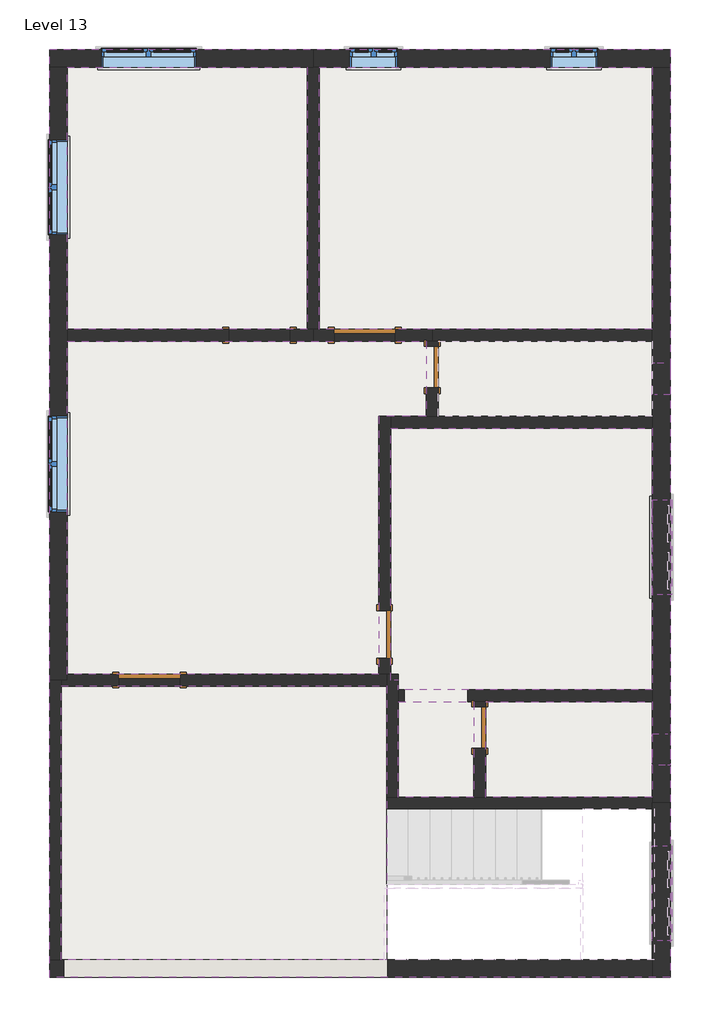
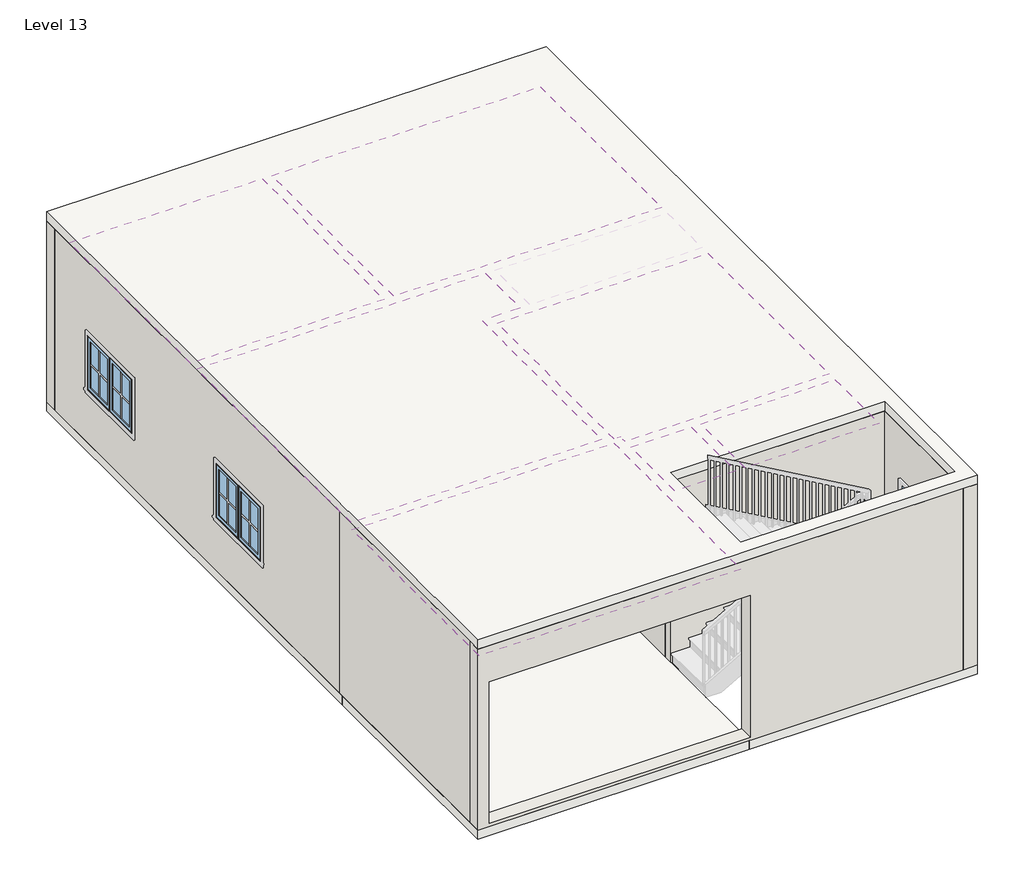
# One storey, part 1 of 2: 27 walls, 13 windows, 7 coverings, 6 doors, 3 slabs.
"""IFC4 building model written with IfcOpenShell, lengths in millimetres."""

from ifc_helpers import new_model, si_unit, frame, origin, place, context, project, spatial, polyline, outline, extrude, faceted_brep, transform, mapped, element, save
from components import door_2908be75, door_9ea4ff49, door_dc34e247, door_b804d09e, fixed_2_415b3208, window_casement_double_3_c417fced, window_casement_double_4_c19c33cb

model = new_model("IFC4")

# Units and contexts
model_context = context("Model", 3, world=origin())
ifc_project = project(units=[si_unit("LENGTHUNIT", "METRE", prefix="MILLI")], contexts=[model_context])

# Site, building, storey
site = spatial("IfcSite", under=ifc_project)
building = spatial("IfcBuilding", under=site)
storey = spatial("IfcBuildingStorey", under=building, Name="Level 13", Elevation=3200.4)

# Coverings
placement = place(None, origin())
element("IfcCovering", 1, ObjectType="2' x 4' ACT System", at=placement, inside=storey, context=model_context, shape_type="SweptSolid", body=[
    extrude(outline(polyline([(-5680.5154463, 2323.8455275), (-5680.5154463, 5678.2330275), (-2607.1154463, 5678.2330275), (-2607.1154463, 2323.8455275), (-5680.5154463, 2323.8455275)])), frame((0.0, 0.0, 5943.6), z_axis=(0.0, 0.0, 1.0), x_axis=(1.0, 0.0, 0.0)), (0.0, 0.0, 1.0), 57.15),
])
element("IfcCovering", 2, ObjectType="2' x 4' ACT System", at=placement, inside=storey, context=model_context, shape_type="SweptSolid", body=[
    extrude(outline(polyline([(-2454.7154463, 2323.8455275), (-2454.7154463, 5678.2330275), (1812.4845537, 5678.2330275), (1812.4845537, 2323.8455275), (-2454.7154463, 2323.8455275)])), frame((0.0, 0.0, 5943.6), z_axis=(0.0, 0.0, 1.0), x_axis=(1.0, 0.0, 0.0)), (0.0, 0.0, 1.0), 57.15),
])
element("IfcCovering", 3, ObjectType="2' x 4' ACT System", at=placement, inside=storey, context=model_context, shape_type="SweptSolid", body=[
    extrude(outline(polyline([(-5680.5154463, -2095.7544725), (-5680.5154463, 2171.4455275), (-1083.1154463, 2171.4455275), (-1083.1154463, 1206.2455275), (-1692.7154463, 1206.2455275), (-1692.7154463, -2095.7544725), (-5680.5154463, -2095.7544725)])), frame((0.0, 0.0, 5943.6), z_axis=(0.0, 0.0, 1.0), x_axis=(1.0, 0.0, 0.0)), (0.0, 0.0, 1.0), 57.15),
])
element("IfcCovering", 4, ObjectType="2' x 4' ACT System", at=placement, inside=storey, context=model_context, shape_type="SweptSolid", body=[
    extrude(outline(polyline([(1812.4845537, 1053.8455275), (1812.4845537, -2298.9544725), (-1438.7154463, -2298.9544725), (-1438.7154463, -2171.9544725), (-1540.3154463, -2171.9544725), (-1540.3154463, 1053.8455275), (1812.4845537, 1053.8455275)])), frame((0.0, 0.0, 5943.6), z_axis=(0.0, 0.0, 1.0), x_axis=(1.0, 0.0, 0.0)), (0.0, 0.0, 1.0), 57.15),
])
element("IfcCovering", 5, ObjectType="2' x 4' ACT System", at=placement, inside=storey, context=model_context, shape_type="SweptSolid", body=[
    extrude(outline(polyline([(1812.4845537, -2451.3544725), (1812.4845537, -3670.5544725), (-321.1154463, -3670.5544725), (-321.1154463, -2451.3544725), (1812.4845537, -2451.3544725)])), frame((0.0, 0.0, 5943.6), z_axis=(0.0, 0.0, 1.0), x_axis=(1.0, 0.0, 0.0)), (0.0, 0.0, 1.0), 57.15),
])
element("IfcCovering", 6, ObjectType="2' x 4' ACT System", at=placement, inside=storey, context=model_context, shape_type="SweptSolid", body=[
    extrude(outline(polyline([(-473.5154463, -2451.3544725), (-473.5154463, -3670.5544725), (-1438.7154463, -3670.5544725), (-1438.7154463, -2451.3544725), (-473.5154463, -2451.3544725)])), frame((0.0, 0.0, 5943.6), z_axis=(0.0, 0.0, 1.0), x_axis=(1.0, 0.0, 0.0)), (0.0, 0.0, 1.0), 57.15),
])
element("IfcCovering", 7, ObjectType="2' x 4' ACT System", at=placement, inside=storey, context=model_context, shape_type="SweptSolid", body=[
    extrude(outline(polyline([(-1591.1154463, -2248.1544725), (-1591.1154463, -5753.3544725), (-5756.7154463, -5753.3544725), (-5756.7154463, -2248.1544725), (-1591.1154463, -2248.1544725)])), frame((0.0, 0.0, 5943.6), z_axis=(0.0, 0.0, 1.0), x_axis=(1.0, 0.0, 0.0)), (0.0, 0.0, 1.0), 57.15),
])

# Doors
door_shape = door_2908be75(model_context)
element("IfcDoor", 8, ObjectType="Single-Flush : 1' 9\"", at=placement, inside=storey, context=model_context, shape_type="MappedRepresentation", body=[
    mapped(door_shape, transform((-397.3154463, -2781.5544725, 3200.4), x_axis=(0.0, 1.0, 0.0), y_axis=(-1.0, 0.0, 0.0), z_axis=(0.0, 0.0, 1.0))),
])
element("IfcDoor", 9, ObjectType="Single-Flush : 1' 9\"", at=placement, inside=storey, context=model_context, shape_type="MappedRepresentation", body=[
    mapped(door_shape, transform((-1006.9154463, 1841.2455275, 3200.4), x_axis=(0.0, 1.0, 0.0), y_axis=(-1.0, 0.0, 0.0), z_axis=(0.0, 0.0, 1.0))),
])
door_2_shape = door_9ea4ff49(model_context)
element("IfcDoor", 10, ObjectType="Single-Flush : 2'0\"", at=placement, inside=storey, context=model_context, shape_type="MappedRepresentation", body=[
    mapped(door_2_shape, transform((-1616.5154463, -1587.7544725, 3200.4), x_axis=(0.0, -1.0, 0.0), y_axis=(1.0, 0.0, 0.0), z_axis=(0.0, 0.0, 1.0))),
])
door_3_shape = door_dc34e247(model_context)
element("IfcDoor", 11, ObjectType="Single-Flush : 2'7\"", at=placement, inside=storey, context=model_context, shape_type="MappedRepresentation", body=[
    mapped(door_3_shape, transform((-4626.4154463, -2171.9544725, 3200.4), x_axis=(-1.0, 0.0, 0.0), y_axis=(0.0, -1.0, 0.0), z_axis=(0.0, 0.0, 1.0))),
])
element("IfcDoor", 12, ObjectType="Single-Flush : 2'7\"", at=placement, inside=storey, context=model_context, shape_type="MappedRepresentation", body=[
    mapped(door_3_shape, transform((-1870.5154463, 2247.6455275, 3200.4), x_axis=(-1.0, 0.0, 0.0), y_axis=(0.0, -1.0, 0.0), z_axis=(0.0, 0.0, 1.0))),
])
door_4_shape = door_b804d09e(model_context)
element("IfcDoor", 13, ObjectType="Single-Flush : 2'7\"", at=placement, inside=storey, context=model_context, shape_type="MappedRepresentation", body=[
    mapped(door_4_shape, transform((-3216.7154463, 2247.6455275, 3200.4), x_axis=(1.0, 0.0, 0.0), y_axis=(0.0, 1.0, 0.0), z_axis=(0.0, 0.0, 1.0))),
])

# Slabs
element("IfcSlab", 14, ObjectType="Generic - 6\"", at=placement, inside=storey, context=model_context, shape_type="SweptSolid", body=[
    extrude(outline(polyline([(-5909.1154463, -2248.1544725), (-5909.1154463, 5906.8330275), (2041.0845537, 5906.8330275), (2041.0845537, -5981.9544725), (-1591.1154463, -5981.9544725), (-1591.1154463, -5753.3544725), (1812.4845537, -5753.3544725), (1812.4845537, -3822.9544725), (-1591.1154463, -3822.9544725), (-1591.1154463, -2248.1544725), (-5756.7154463, -2248.1544725), (-5909.1154463, -2248.1544725)])), frame((0.0, 0.0, 3048.0), z_axis=(0.0, 0.0, 1.0), x_axis=(1.0, 0.0, 0.0)), (0.0, 0.0, 1.0), 152.4),
])
element("IfcSlab", 15, ObjectType="Generic - 6\"", at=placement, inside=storey, context=model_context, shape_type="SweptSolid", body=[
    extrude(outline(polyline([(-1591.1154463, -2248.1544725), (-1591.1154463, -5981.9544725), (-5909.1154463, -5981.9544725), (-5909.1154463, -2248.1544725), (-1591.1154463, -2248.1544725)])), frame((0.0, 0.0, 3048.0), z_axis=(0.0, 0.0, 1.0), x_axis=(1.0, 0.0, 0.0)), (0.0, 0.0, 1.0), 152.4),
])
element("IfcSlab", 16, ObjectType="Generic - 6\"", at=placement, inside=storey, context=model_context, shape_type="SweptSolid", body=[
    extrude(outline(polyline([(2041.0845537, 5906.8330275), (2041.0845537, -5981.9544725), (-5909.1154463, -5981.9544725), (-5909.1154463, 5906.8330275), (2041.0845537, 5906.8330275)]), holes=[polyline([(1812.4845537, -3822.9544725), (-1591.1154463, -3822.9544725), (-1591.1154463, -5753.3544725), (1812.4845537, -5753.3544725), (1812.4845537, -3822.9544725)])]), frame((0.0, 0.0, 6248.4), z_axis=(0.0, 0.0, 1.0), x_axis=(1.0, 0.0, 0.0)), (0.0, 0.0, 1.0), 152.4),
])

# Walls
element("IfcWall", 17, ObjectType="Generic - 6\"", at=placement, inside=storey, context=model_context, shape_type="Brep", body=[
    faceted_brep([(-5909.1154463, -2171.9544725, 3200.4), (-5909.1154463, -5753.3544725, 3200.4), (-5909.1154463, -5753.3544725, 6248.4), (-5909.1154463, -2171.9544725, 6248.4), (-5756.7154463, -2171.9544725, 3200.4), (-5756.7154463, -2171.9544725, 6248.4), (-5756.7154463, -2248.1544725, 6248.4), (-5756.7154463, -5753.3544725, 6248.4), (-5756.7154463, -5753.3544725, 3200.4), (-5756.7154463, -2248.1544725, 3200.4)], [[[0, 1, 2, 3]], [[4, 5, 6, 7, 8, 9]], [[1, 0, 4, 9, 8]], [[3, 2, 7, 6, 5]], [[0, 3, 5, 4]], [[2, 1, 8, 7]]]),
])
element("IfcWall", 18, ObjectType="Generic - 6\"", at=placement, inside=storey, context=model_context, shape_type="Brep", body=[
    faceted_brep([(1812.4845537, -3670.5544725, 3200.4), (-321.1154463, -3670.5544725, 3200.4), (-473.5154463, -3670.5544725, 3200.4), (-1438.7154463, -3670.5544725, 3200.4), (-1591.1154463, -3670.5544725, 3200.4), (-1591.1154463, -3670.5544725, 6248.4), (-1438.7154463, -3670.5544725, 6248.4), (-473.5154463, -3670.5544725, 6248.4), (-321.1154463, -3670.5544725, 6248.4), (1812.4845537, -3670.5544725, 6248.4), (1812.4845537, -3822.9544725, 3200.4), (1812.4845537, -3822.9544725, 6248.4), (-1591.1154463, -3822.9544725, 6248.4), (-1591.1154463, -3822.9544725, 3200.4), (1812.4845537, -3746.7544725, 3200.4), (1812.4845537, -3746.7544725, 6248.4)], [[[0, 1, 2, 3, 4, 5, 6, 7, 8, 9]], [[10, 11, 12, 13]], [[4, 3, 2, 1, 0, 14, 10, 13]], [[9, 8, 7, 6, 5, 12, 11, 15]], [[5, 4, 13, 12]], [[0, 9, 15, 11, 10, 14]]]),
])
element("IfcWall", 19, ObjectType="Generic - 6\"", at=placement, inside=storey, context=model_context, shape_type="Brep", body=[
    faceted_brep([(-1438.7154463, -3670.5544725, 3200.4), (-1438.7154463, -2451.3544725, 3200.4), (-1438.7154463, -2298.9544725, 3200.4), (-1438.7154463, -2095.7544725, 3200.4), (-1438.7154463, -2095.7544725, 6248.4), (-1438.7154463, -2298.9544725, 6248.4), (-1438.7154463, -2451.3544725, 6248.4), (-1438.7154463, -3670.5544725, 6248.4), (-1591.1154463, -3670.5544725, 3200.4), (-1591.1154463, -3670.5544725, 6248.4), (-1591.1154463, -2248.1544725, 6248.4), (-1591.1154463, -2171.9544725, 6248.4), (-1591.1154463, -2095.7544725, 6248.4), (-1591.1154463, -2095.7544725, 3200.4), (-1591.1154463, -2171.9544725, 3200.4), (-1591.1154463, -2248.1544725, 3200.4), (-1540.3154463, -2095.7544725, 3200.4), (-1540.3154463, -2095.7544725, 6248.4)], [[[0, 1, 2, 3, 4, 5, 6, 7]], [[8, 9, 10, 11, 12, 13, 14, 15]], [[3, 2, 1, 0, 8, 15, 14, 13, 16]], [[7, 6, 5, 4, 17, 12, 11, 10, 9]], [[0, 7, 9, 8]], [[4, 3, 16, 13, 12, 17]]]),
])
element("IfcWall", 20, ObjectType="Generic - 6\"", at=placement, inside=storey, context=model_context, shape_type="Brep", body=[
    faceted_brep([(-5020.1154463, -2095.7544725, 5334.0), (-5020.1154463, -2095.7544725, 3200.4), (-5680.5154463, -2095.7544725, 3200.4), (-5680.5154463, -2095.7544725, 6248.4), (-1692.7154463, -2095.7544725, 6248.4), (-1591.1154463, -2095.7544725, 6248.4), (-1591.1154463, -2095.7544725, 3200.4), (-1692.7154463, -2095.7544725, 3200.4), (-4232.7154463, -2095.7544725, 3200.4), (-4232.7154463, -2095.7544725, 5334.0), (-5756.7154463, -2248.1544725, 3200.4), (-5020.1154463, -2248.1544725, 3200.4), (-5020.1154463, -2248.1544725, 5334.0), (-4232.7154463, -2248.1544725, 5334.0), (-4232.7154463, -2248.1544725, 3200.4), (-1591.1154463, -2248.1544725, 3200.4), (-1591.1154463, -2248.1544725, 6248.4), (-5756.7154463, -2248.1544725, 6248.4), (-5756.7154463, -2171.9544725, 3200.4), (-5680.5154463, -2171.9544725, 3200.4), (-5680.5154463, -2171.9544725, 6248.4), (-5756.7154463, -2171.9544725, 6248.4)], [[[0, 1, 2, 3, 4, 5, 6, 7, 8, 9]], [[10, 11, 12, 13, 14, 15, 16, 17]], [[2, 1, 11, 10, 18, 19]], [[8, 7, 6, 15, 14]], [[5, 4, 3, 20, 21, 17, 16]], [[3, 2, 19, 20]], [[19, 18, 21, 20]], [[18, 10, 17, 21]], [[6, 5, 16, 15]], [[12, 11, 1, 0]], [[13, 12, 0, 9]], [[14, 13, 9, 8]]]),
])
element("IfcWall", 21, ObjectType="Generic - 6\"", at=placement, inside=storey, context=model_context, shape_type="Brep", body=[
    faceted_brep([(1812.4845537, -2451.3544725, 3200.4), (1812.4845537, -2451.3544725, 6248.4), (-321.1154463, -2451.3544725, 6248.4), (-473.5154463, -2451.3544725, 6248.4), (-1438.7154463, -2451.3544725, 6248.4), (-1438.7154463, -2451.3544725, 3200.4), (-1367.0206652, -2451.3544725, 3200.4), (-1367.0206652, -2451.3544725, 5638.8), (-547.4818767, -2451.3544725, 5638.8), (-547.4818767, -2451.3544725, 3200.4), (-473.5154463, -2451.3544725, 3200.4), (-321.1154463, -2451.3544725, 3200.4), (1812.4845537, -2298.9544725, 6248.4), (1812.4845537, -2298.9544725, 3200.4), (-547.4818767, -2298.9544725, 3200.4), (-547.4818767, -2298.9544725, 5638.8), (-1367.0206652, -2298.9544725, 5638.8), (-1367.0206652, -2298.9544725, 3200.4), (-1438.7154463, -2298.9544725, 3200.4), (-1438.7154463, -2298.9544725, 6248.4)], [[[0, 1, 2, 3, 4, 5, 6, 7, 8, 9, 10, 11]], [[12, 13, 14, 15, 16, 17, 18, 19]], [[5, 18, 17, 6]], [[13, 0, 11, 10, 9, 14]], [[4, 3, 2, 1, 12, 19]], [[1, 0, 13, 12]], [[5, 4, 19, 18]], [[7, 16, 15, 8]], [[16, 7, 6, 17]], [[8, 15, 14, 9]]]),
])
element("IfcWall", 22, ObjectType="Generic - 6\"", at=placement, inside=storey, context=model_context, shape_type="SweptSolid", body=[
    extrude(outline(polyline([(-2451.3544725, 3200.4), (-2514.8544725, 3200.4), (-2514.8544725, 5334.0), (-3048.2544725, 5334.0), (-3048.2544725, 3200.4), (-3670.5544725, 3200.4), (-3670.5544725, 6248.4), (-2451.3544725, 6248.4), (-2451.3544725, 3200.4)])), frame((-473.5154463, 0.0, 0.0), z_axis=(1.0, 0.0, 0.0), x_axis=(0.0, 1.0, 0.0)), (0.0, 0.0, 1.0), 152.4),
])
element("IfcWall", 23, ObjectType="Generic - 6\"", at=placement, inside=storey, context=model_context, shape_type="Brep", body=[
    faceted_brep([(-1540.3154463, -2095.7544725, 3200.4), (-1540.3154463, -1892.5544725, 3200.4), (-1540.3154463, -1892.5544725, 5334.0), (-1540.3154463, -1282.9544725, 5334.0), (-1540.3154463, -1282.9544725, 3200.4), (-1540.3154463, 1053.8455275, 3200.4), (-1540.3154463, 1206.2455275, 3200.4), (-1540.3154463, 1206.2455275, 6248.4), (-1540.3154463, 1053.8455275, 6248.4), (-1540.3154463, -2095.7544725, 6248.4), (-1692.7154463, -1892.5544725, 5334.0), (-1692.7154463, -1892.5544725, 3200.4), (-1692.7154463, -2095.7544725, 3200.4), (-1692.7154463, -2095.7544725, 6248.4), (-1692.7154463, 1206.2455275, 6248.4), (-1692.7154463, 1206.2455275, 3200.4), (-1692.7154463, -1282.9544725, 3200.4), (-1692.7154463, -1282.9544725, 5334.0), (-1591.1154463, -2095.7544725, 3200.4), (-1591.1154463, -2095.7544725, 6248.4)], [[[0, 1, 2, 3, 4, 5, 6, 7, 8, 9]], [[10, 11, 12, 13, 14, 15, 16, 17]], [[16, 15, 6, 5, 4]], [[12, 11, 1, 0, 18]], [[9, 8, 7, 14, 13, 19]], [[0, 9, 19, 13, 12, 18]], [[7, 6, 15, 14]], [[2, 1, 11, 10]], [[3, 2, 10, 17]], [[4, 3, 17, 16]]]),
])
element("IfcWall", 24, ObjectType="Generic - 6\"", at=placement, inside=storey, context=model_context, shape_type="Brep", body=[
    faceted_brep([(-1540.3154463, 1053.8455275, 3200.4), (1812.4845537, 1053.8455275, 3200.4), (1812.4845537, 1053.8455275, 6248.4), (-1540.3154463, 1053.8455275, 6248.4), (-1540.3154463, 1206.2455275, 3200.4), (-1540.3154463, 1206.2455275, 6248.4), (-1083.1154463, 1206.2455275, 6248.4), (-930.7154463, 1206.2455275, 6248.4), (1812.4845537, 1206.2455275, 6248.4), (1812.4845537, 1206.2455275, 3200.4), (-930.7154463, 1206.2455275, 3200.4), (-1083.1154463, 1206.2455275, 3200.4)], [[[0, 1, 2, 3]], [[4, 5, 6, 7, 8, 9, 10, 11]], [[1, 0, 4, 11, 10, 9]], [[3, 2, 8, 7, 6, 5]], [[0, 3, 5, 4]], [[2, 1, 9, 8]]]),
])
element("IfcWall", 25, ObjectType="Generic - 6\"", at=placement, inside=storey, context=model_context, shape_type="Brep", body=[
    faceted_brep([(-930.7154463, 2107.9455275, 5334.0), (-930.7154463, 2107.9455275, 3200.4), (-930.7154463, 2171.4455275, 3200.4), (-930.7154463, 2171.4455275, 6248.4), (-930.7154463, 1206.2455275, 6248.4), (-930.7154463, 1206.2455275, 3200.4), (-930.7154463, 1574.5455275, 3200.4), (-930.7154463, 1574.5455275, 5334.0), (-1083.1154463, 2171.4455275, 3200.4), (-1083.1154463, 2107.9455275, 3200.4), (-1083.1154463, 2107.9455275, 5334.0), (-1083.1154463, 1574.5455275, 5334.0), (-1083.1154463, 1574.5455275, 3200.4), (-1083.1154463, 1206.2455275, 3200.4), (-1083.1154463, 1206.2455275, 6248.4), (-1083.1154463, 2171.4455275, 6248.4), (-1006.9154463, 2171.4455275, 3200.4), (-1006.9154463, 2171.4455275, 6248.4)], [[[0, 1, 2, 3, 4, 5, 6, 7]], [[8, 9, 10, 11, 12, 13, 14, 15]], [[6, 5, 13, 12]], [[2, 1, 9, 8, 16]], [[4, 3, 17, 15, 14]], [[5, 4, 14, 13]], [[10, 9, 1, 0]], [[11, 10, 0, 7]], [[12, 11, 7, 6]], [[3, 2, 16, 8, 15, 17]]]),
])
element("IfcWall", 26, ObjectType="Generic - 6\"", at=placement, inside=storey, context=model_context, shape_type="Brep", body=[
    faceted_brep([(1812.4845537, 2323.8455275, 3200.4), (-1006.9154463, 2323.8455275, 3200.4), (-1006.9154463, 2323.8455275, 6248.4), (1812.4845537, 2323.8455275, 6248.4), (1812.4845537, 2171.4455275, 3200.4), (1812.4845537, 2171.4455275, 6248.4), (-930.7154463, 2171.4455275, 6248.4), (-1006.9154463, 2171.4455275, 6248.4), (-1006.9154463, 2171.4455275, 3200.4), (-930.7154463, 2171.4455275, 3200.4)], [[[0, 1, 2, 3]], [[4, 5, 6, 7, 8, 9]], [[1, 0, 4, 9, 8]], [[2, 1, 8, 7]], [[3, 2, 7, 6, 5]], [[0, 3, 5, 4]]]),
])
element("IfcWall", 27, ObjectType="Generic - 6\"", at=placement, inside=storey, context=model_context, shape_type="Brep", body=[
    faceted_brep([(-2607.1154463, 5678.2330275, 3200.4), (-2607.1154463, 2323.8455275, 3200.4), (-2607.1154463, 2323.8455275, 6248.4), (-2607.1154463, 5678.2330275, 6248.4), (-2454.7154463, 5678.2330275, 3200.4), (-2454.7154463, 5678.2330275, 6248.4), (-2454.7154463, 2323.8455275, 6248.4), (-2454.7154463, 2323.8455275, 3200.4), (-2530.9154463, 5678.2330275, 3200.4), (-2530.9154463, 2323.8455275, 3200.4), (-2530.9154463, 2323.8455275, 6248.4), (-2530.9154463, 5678.2330275, 6248.4)], [[[0, 1, 2, 3]], [[4, 5, 6, 7]], [[1, 0, 8, 4, 7, 9]], [[3, 2, 10, 6, 5, 11]], [[0, 3, 11, 5, 4, 8]], [[2, 1, 9, 7, 6, 10]]]),
])
element("IfcWall", 28, ObjectType="Generic - 6\"", at=placement, inside=storey, context=model_context, shape_type="Brep", body=[
    faceted_brep([(-2530.9154463, 2323.8455275, 3200.4), (-2607.1154463, 2323.8455275, 3200.4), (-2823.0154463, 2323.8455275, 3200.4), (-2823.0154463, 2323.8455275, 5334.0), (-3610.4154463, 2323.8455275, 5334.0), (-3610.4154463, 2323.8455275, 3200.4), (-5680.5154463, 2323.8455275, 3200.4), (-5680.5154463, 2323.8455275, 6248.4), (-2607.1154463, 2323.8455275, 6248.4), (-2530.9154463, 2323.8455275, 6248.4), (-2823.0154463, 2171.4455275, 5334.0), (-2823.0154463, 2171.4455275, 3200.4), (-2530.9154463, 2171.4455275, 3200.4), (-2530.9154463, 2171.4455275, 6248.4), (-5680.5154463, 2171.4455275, 6248.4), (-5680.5154463, 2171.4455275, 3200.4), (-3610.4154463, 2171.4455275, 3200.4), (-3610.4154463, 2171.4455275, 5334.0)], [[[0, 1, 2, 3, 4, 5, 6, 7, 8, 9]], [[10, 11, 12, 13, 14, 15, 16, 17]], [[16, 15, 6, 5]], [[12, 11, 2, 1, 0]], [[9, 8, 7, 14, 13]], [[0, 9, 13, 12]], [[7, 6, 15, 14]], [[5, 4, 17, 16]], [[4, 3, 10, 17]], [[3, 2, 11, 10]]]),
])
element("IfcWall", 29, ObjectType="Generic - 6\"", at=placement, inside=storey, context=model_context, shape_type="Brep", body=[
    faceted_brep([(-2264.2154463, 2323.8455275, 5334.0), (-2264.2154463, 2323.8455275, 3200.4), (-2454.7154463, 2323.8455275, 3200.4), (-2530.9154463, 2323.8455275, 3200.4), (-2530.9154463, 2323.8455275, 6248.4), (-2454.7154463, 2323.8455275, 6248.4), (-1006.9154463, 2323.8455275, 6248.4), (-1006.9154463, 2323.8455275, 3200.4), (-1476.8154463, 2323.8455275, 3200.4), (-1476.8154463, 2323.8455275, 5334.0), (-2530.9154463, 2171.4455275, 3200.4), (-2264.2154463, 2171.4455275, 3200.4), (-2264.2154463, 2171.4455275, 5334.0), (-1476.8154463, 2171.4455275, 5334.0), (-1476.8154463, 2171.4455275, 3200.4), (-1083.1154463, 2171.4455275, 3200.4), (-1006.9154463, 2171.4455275, 3200.4), (-1006.9154463, 2171.4455275, 6248.4), (-1083.1154463, 2171.4455275, 6248.4), (-2530.9154463, 2171.4455275, 6248.4)], [[[0, 1, 2, 3, 4, 5, 6, 7, 8, 9]], [[10, 11, 12, 13, 14, 15, 16, 17, 18, 19]], [[8, 7, 16, 15, 14]], [[3, 2, 1, 11, 10]], [[4, 3, 10, 19]], [[6, 5, 4, 19, 18, 17]], [[7, 6, 17, 16]], [[14, 13, 9, 8]], [[13, 12, 0, 9]], [[12, 11, 1, 0]]]),
])
element("IfcWall", 30, ObjectType="Generic - 6\"", at=placement, inside=storey, context=model_context, shape_type="SweptSolid", body=[
    extrude(outline(polyline([(-5680.5154463, -2095.7544725), (-1692.7154463, -2095.7544725), (-1692.7154463, -2171.9544725), (-1591.1154463, -2171.9544725), (-1591.1154463, -2248.1544725), (-5756.7154463, -2248.1544725), (-5756.7154463, -2171.9544725), (-5680.5154463, -2171.9544725), (-5680.5154463, -2095.7544725)])), frame((0.0, 0.0, 3200.4), z_axis=(0.0, 0.0, 1.0), x_axis=(1.0, 0.0, 0.0)), (0.0, 0.0, 1.0), 3048.0),
])
element("IfcWall", 31, ObjectType="Generic - 6\"", at=placement, inside=storey, context=model_context, shape_type="Brep", body=[
    faceted_brep([(-2607.1154463, 5678.2330275, 3200.4), (-2607.1154463, 2323.8455275, 3200.4), (-2607.1154463, 2323.8455275, 6248.4), (-2607.1154463, 5678.2330275, 6248.4), (-2454.7154463, 5678.2330275, 3200.4), (-2454.7154463, 5678.2330275, 6248.4), (-2454.7154463, 2323.8455275, 6248.4), (-2454.7154463, 2323.8455275, 3200.4), (-2530.9154463, 5678.2330275, 3200.4), (-2530.9154463, 2323.8455275, 3200.4), (-2530.9154463, 2323.8455275, 6248.4), (-2530.9154463, 5678.2330275, 6248.4)], [[[0, 1, 2, 3]], [[4, 5, 6, 7]], [[1, 0, 8, 4, 7, 9]], [[3, 2, 10, 6, 5, 11]], [[0, 3, 11, 5, 4, 8]], [[2, 1, 9, 7, 6, 10]]]),
])
element("IfcWall", 32, ObjectType="Generic - 6\"", at=placement, inside=storey, context=model_context, shape_type="Brep", body=[
    faceted_brep([(-2530.9154463, 2323.8455275, 3200.4), (-2607.1154463, 2323.8455275, 3200.4), (-5680.5154463, 2323.8455275, 3200.4), (-5680.5154463, 2323.8455275, 6248.4), (-2607.1154463, 2323.8455275, 6248.4), (-2530.9154463, 2323.8455275, 6248.4), (-2530.9154463, 2171.4455275, 3200.4), (-2530.9154463, 2171.4455275, 6248.4), (-5680.5154463, 2171.4455275, 6248.4), (-5680.5154463, 2171.4455275, 3200.4)], [[[0, 1, 2, 3, 4, 5]], [[6, 7, 8, 9]], [[2, 1, 0, 6, 9]], [[5, 4, 3, 8, 7]], [[0, 5, 7, 6]], [[3, 2, 9, 8]]]),
])
element("IfcWall", 33, ObjectType="Generic - 6\"", at=placement, inside=storey, context=model_context, shape_type="Brep", body=[
    faceted_brep([(-1006.9154463, 2323.8455275, 3200.4), (-2454.7154463, 2323.8455275, 3200.4), (-2530.9154463, 2323.8455275, 3200.4), (-2530.9154463, 2323.8455275, 6248.4), (-2454.7154463, 2323.8455275, 6248.4), (-1006.9154463, 2323.8455275, 6248.4), (-1006.9154463, 2171.4455275, 3200.4), (-1006.9154463, 2171.4455275, 6248.4), (-1083.1154463, 2171.4455275, 6248.4), (-2530.9154463, 2171.4455275, 6248.4), (-2530.9154463, 2171.4455275, 3200.4), (-1083.1154463, 2171.4455275, 3200.4)], [[[0, 1, 2, 3, 4, 5]], [[6, 7, 8, 9, 10, 11]], [[2, 1, 0, 6, 11, 10]], [[3, 2, 10, 9]], [[5, 4, 3, 9, 8, 7]], [[0, 5, 7, 6]]]),
])
element("IfcWall", 34, ObjectType="Generic - 9\"", at=placement, inside=storey, context=model_context, shape_type="Brep", body=[
    faceted_brep([(-5909.1154463, 5678.2330275, 3200.4), (-5680.5154463, 5678.2330275, 3200.4), (-2607.1154463, 5678.2330275, 3200.4), (-2530.9154463, 5678.2330275, 3200.4), (-2530.9154463, 5678.2330275, 6248.4), (-2607.1154463, 5678.2330275, 6248.4), (-5680.5154463, 5678.2330275, 6248.4), (-5909.1154463, 5678.2330275, 6248.4), (-4029.5154463, 5678.2330275, 5029.2), (-4029.5154463, 5678.2330275, 4114.8), (-5248.7154463, 5678.2330275, 4114.8), (-5248.7154463, 5678.2330275, 5029.2), (-5909.1154463, 5906.8330275, 3200.4), (-5909.1154463, 5906.8330275, 6248.4), (-2530.9154463, 5906.8330275, 6248.4), (-2530.9154463, 5906.8330275, 3200.4), (-4029.5154463, 5906.8330275, 5029.2), (-5248.7154463, 5906.8330275, 5029.2), (-5248.7154463, 5906.8330275, 4114.8), (-4029.5154463, 5906.8330275, 4114.8)], [[[0, 1, 2, 3, 4, 5, 6, 7], [8, 9, 10, 11]], [[12, 13, 14, 15], [16, 17, 18, 19]], [[3, 2, 1, 0, 12, 15]], [[4, 3, 15, 14]], [[7, 6, 5, 4, 14, 13]], [[0, 7, 13, 12]], [[9, 8, 16, 19]], [[10, 9, 19, 18]], [[11, 10, 18, 17]], [[8, 11, 17, 16]]]),
])
element("IfcWall", 35, ObjectType="Generic - 9\"", at=placement, inside=storey, context=model_context, shape_type="Brep", body=[
    faceted_brep([(1812.4845537, 5678.2330275, 3200.4), (1812.4845537, 2323.8455275, 3200.4), (1812.4845537, 2171.4455275, 3200.4), (1812.4845537, 1206.2455275, 3200.4), (1812.4845537, 1053.8455275, 3200.4), (1812.4845537, -2298.9544725, 3200.4), (1812.4845537, -2451.3544725, 3200.4), (1812.4845537, -3670.5544725, 3200.4), (1812.4845537, -3746.7544725, 3200.4), (1812.4845537, -3746.7544725, 6248.4), (1812.4845537, -3670.5544725, 6248.4), (1812.4845537, -2451.3544725, 6248.4), (1812.4845537, -2298.9544725, 6248.4), (1812.4845537, 1053.8455275, 6248.4), (1812.4845537, 1206.2455275, 6248.4), (1812.4845537, 2171.4455275, 6248.4), (1812.4845537, 2323.8455275, 6248.4), (1812.4845537, 5678.2330275, 6248.4), (1812.4845537, -1079.7544725, 5334.0), (1812.4845537, -1079.7544725, 4419.6), (1812.4845537, 139.4455275, 4419.6), (1812.4845537, 139.4455275, 5334.0), (1812.4845537, -3264.1544725, 5638.8), (1812.4845537, -3264.1544725, 5029.2), (1812.4845537, -2857.7544725, 5029.2), (1812.4845537, -2857.7544725, 5638.8), (1812.4845537, 1892.0455275, 5638.8), (1812.4845537, 1485.6455275, 5638.8), (1812.4845537, 1485.6455275, 5029.2), (1812.4845537, 1892.0455275, 5029.2), (2041.0845537, 5678.2330275, 3200.4), (2041.0845537, 5678.2330275, 6248.4), (2041.0845537, -3746.7544725, 6248.4), (2041.0845537, -3746.7544725, 3200.4), (2041.0845537, -1079.7544725, 5334.0), (2041.0845537, 139.4455275, 5334.0), (2041.0845537, 139.4455275, 4419.6), (2041.0845537, -1079.7544725, 4419.6), (2041.0845537, -3264.1544725, 5638.8), (2041.0845537, -2857.7544725, 5638.8), (2041.0845537, -2857.7544725, 5029.2), (2041.0845537, -3264.1544725, 5029.2), (2041.0845537, 1892.0455275, 5638.8), (2041.0845537, 1892.0455275, 5029.2), (2041.0845537, 1485.6455275, 5029.2), (2041.0845537, 1485.6455275, 5638.8)], [[[0, 1, 2, 3, 4, 5, 6, 7, 8, 9, 10, 11, 12, 13, 14, 15, 16, 17], [18, 19, 20, 21], [22, 23, 24, 25], [26, 27, 28, 29]], [[30, 31, 32, 33], [34, 35, 36, 37], [38, 39, 40, 41], [42, 43, 44, 45]], [[8, 7, 6, 5, 4, 3, 2, 1, 0, 30, 33]], [[9, 8, 33, 32]], [[17, 16, 15, 14, 13, 12, 11, 10, 9, 32, 31]], [[0, 17, 31, 30]], [[19, 18, 34, 37]], [[20, 19, 37, 36]], [[21, 20, 36, 35]], [[18, 21, 35, 34]], [[23, 22, 38, 41]], [[24, 23, 41, 40]], [[25, 24, 40, 39]], [[22, 25, 39, 38]], [[43, 42, 26, 29]], [[44, 43, 29, 28]], [[45, 44, 28, 27]], [[42, 45, 27, 26]]]),
])
element("IfcWall", 36, ObjectType="Generic - 9\"", at=placement, inside=storey, context=model_context, shape_type="Brep", body=[
    faceted_brep([(1812.4845537, -5753.3544725, 3200.4), (-5756.7154463, -5753.3544725, 3200.4), (-5909.1154463, -5753.3544725, 3200.4), (-5909.1154463, -5753.3544725, 6248.4), (-5756.7154463, -5753.3544725, 6248.4), (1812.4845537, -5753.3544725, 6248.4), (-1576.8982041, -5753.3544725, 5638.8), (-5729.1673724, -5753.3544725, 5638.8), (-5729.1673724, -5753.3544725, 3251.2), (-1576.8982041, -5753.3544725, 3251.2), (-5909.1154463, -5981.9544725, 3200.4), (1812.4845537, -5981.9544725, 3200.4), (1812.4845537, -5981.9544725, 6248.4), (-5909.1154463, -5981.9544725, 6248.4), (-5729.1673724, -5981.9544725, 5638.8), (-1576.8982041, -5981.9544725, 5638.8), (-1576.8982041, -5981.9544725, 3251.2), (-5729.1673724, -5981.9544725, 3251.2)], [[[0, 1, 2, 3, 4, 5], [6, 7, 8, 9]], [[10, 11, 12, 13], [14, 15, 16, 17]], [[2, 1, 0, 11, 10]], [[5, 4, 3, 13, 12]], [[0, 5, 12, 11]], [[6, 15, 14, 7]], [[8, 17, 16, 9]], [[15, 6, 9, 16]], [[7, 14, 17, 8]], [[3, 2, 10, 13]]]),
])
element("IfcWall", 37, ObjectType="Generic - 9\"", at=placement, inside=storey, context=model_context, shape_type="Brep", body=[
    faceted_brep([(-5909.1154463, 5678.2330275, 3200.4), (-5909.1154463, -2171.9544725, 3200.4), (-5909.1154463, -2171.9544725, 6248.4), (-5909.1154463, 5678.2330275, 6248.4), (-5909.1154463, 4751.1330275, 5029.2), (-5909.1154463, 3531.9330275, 5029.2), (-5909.1154463, 3531.9330275, 4114.8), (-5909.1154463, 4751.1330275, 4114.8), (-5909.1154463, 1206.2455275, 5029.2), (-5909.1154463, -12.9544725, 5029.2), (-5909.1154463, -12.9544725, 4114.8), (-5909.1154463, 1206.2455275, 4114.8), (-5680.5154463, 5678.2330275, 3200.4), (-5680.5154463, 5678.2330275, 6248.4), (-5680.5154463, 2323.8455275, 6248.4), (-5680.5154463, 2171.4455275, 6248.4), (-5680.5154463, -2095.7544725, 6248.4), (-5680.5154463, -2171.9544725, 6248.4), (-5680.5154463, -2171.9544725, 3200.4), (-5680.5154463, -2095.7544725, 3200.4), (-5680.5154463, 2171.4455275, 3200.4), (-5680.5154463, 2323.8455275, 3200.4), (-5680.5154463, 4751.1330275, 5029.2), (-5680.5154463, 4751.1330275, 4114.8), (-5680.5154463, 3531.9330275, 4114.8), (-5680.5154463, 3531.9330275, 5029.2), (-5680.5154463, 1206.2455275, 5029.2), (-5680.5154463, 1206.2455275, 4114.8), (-5680.5154463, -12.9544725, 4114.8), (-5680.5154463, -12.9544725, 5029.2), (-5756.7154463, -2171.9544725, 3200.4), (-5756.7154463, -2171.9544725, 6248.4)], [[[0, 1, 2, 3], [4, 5, 6, 7], [8, 9, 10, 11]], [[12, 13, 14, 15, 16, 17, 18, 19, 20, 21], [22, 23, 24, 25], [26, 27, 28, 29]], [[1, 0, 12, 21, 20, 19, 18, 30]], [[2, 1, 30, 18, 17, 31]], [[3, 2, 31, 17, 16, 15, 14, 13]], [[0, 3, 13, 12]], [[23, 22, 4, 7]], [[24, 23, 7, 6]], [[25, 24, 6, 5]], [[22, 25, 5, 4]], [[27, 26, 8, 11]], [[28, 27, 11, 10]], [[29, 28, 10, 9]], [[26, 29, 9, 8]]]),
])
element("IfcWall", 38, ObjectType="Generic - 9\"", at=placement, inside=storey, context=model_context, shape_type="Brep", body=[
    faceted_brep([(-2530.9154463, 5678.2330275, 3200.4), (-2454.7154463, 5678.2330275, 3200.4), (1812.4845537, 5678.2330275, 3200.4), (2041.0845537, 5678.2330275, 3200.4), (2041.0845537, 5678.2330275, 6248.4), (1812.4845537, 5678.2330275, 6248.4), (-2454.7154463, 5678.2330275, 6248.4), (-2530.9154463, 5678.2330275, 6248.4), (-1451.4154463, 5678.2330275, 5029.2), (-1451.4154463, 5678.2330275, 4114.8), (-2061.0154463, 5678.2330275, 4114.8), (-2061.0154463, 5678.2330275, 5029.2), (1113.9845537, 5678.2330275, 5029.2), (1113.9845537, 5678.2330275, 4114.8), (504.3845537, 5678.2330275, 4114.8), (504.3845537, 5678.2330275, 5029.2), (-2530.9154463, 5906.8330275, 3200.4), (-2530.9154463, 5906.8330275, 6248.4), (2041.0845537, 5906.8330275, 6248.4), (2041.0845537, 5906.8330275, 3200.4), (-1451.4154463, 5906.8330275, 5029.2), (-2061.0154463, 5906.8330275, 5029.2), (-2061.0154463, 5906.8330275, 4114.8), (-1451.4154463, 5906.8330275, 4114.8), (1113.9845537, 5906.8330275, 5029.2), (504.3845537, 5906.8330275, 5029.2), (504.3845537, 5906.8330275, 4114.8), (1113.9845537, 5906.8330275, 4114.8)], [[[0, 1, 2, 3, 4, 5, 6, 7], [8, 9, 10, 11], [12, 13, 14, 15]], [[16, 17, 18, 19], [20, 21, 22, 23], [24, 25, 26, 27]], [[3, 2, 1, 0, 16, 19]], [[7, 6, 5, 4, 18, 17]], [[0, 7, 17, 16]], [[4, 3, 19, 18]], [[8, 11, 21, 20]], [[11, 10, 22, 21]], [[10, 9, 23, 22]], [[9, 8, 20, 23]], [[12, 15, 25, 24]], [[15, 14, 26, 25]], [[14, 13, 27, 26]], [[13, 12, 24, 27]]]),
])
element("IfcWall", 39, ObjectType="Generic - 9\"", at=placement, inside=storey, context=model_context, shape_type="Brep", body=[
    faceted_brep([(1812.4845537, -3746.7544725, 3200.4), (1812.4845537, -3822.9544725, 3200.4), (1812.4845537, -5753.3544725, 3200.4), (1812.4845537, -5981.9544725, 3200.4), (1812.4845537, -5981.9544725, 6248.4), (1812.4845537, -5753.3544725, 6248.4), (1812.4845537, -3822.9544725, 6248.4), (1812.4845537, -3746.7544725, 6248.4), (1812.4845537, -5512.0544725, 5334.0), (1812.4845537, -5512.0544725, 4419.6), (1812.4845537, -4292.8544725, 4419.6), (1812.4845537, -4292.8544725, 5334.0), (2041.0845537, -3746.7544725, 3200.4), (2041.0845537, -3746.7544725, 6248.4), (2041.0845537, -5981.9544725, 6248.4), (2041.0845537, -5981.9544725, 3200.4), (2041.0845537, -5512.0544725, 5334.0), (2041.0845537, -4292.8544725, 5334.0), (2041.0845537, -4292.8544725, 4419.6), (2041.0845537, -5512.0544725, 4419.6)], [[[0, 1, 2, 3, 4, 5, 6, 7], [8, 9, 10, 11]], [[12, 13, 14, 15], [16, 17, 18, 19]], [[3, 2, 1, 0, 12, 15]], [[7, 6, 5, 4, 14, 13]], [[0, 7, 13, 12]], [[4, 3, 15, 14]], [[8, 11, 17, 16]], [[11, 10, 18, 17]], [[10, 9, 19, 18]], [[9, 8, 16, 19]]]),
])
element("IfcWall", 40, ObjectType="Generic - 9\"", at=placement, inside=storey, context=model_context, shape_type="SweptSolid", body=[
    extrude(outline(polyline([(3200.4, -5680.5154463), (3200.4, -2607.1154463), (6248.4, -2607.1154463), (6248.4, -5680.5154463), (3200.4, -5680.5154463)]), holes=[polyline([(5029.2, -4029.5154463), (4114.8, -4029.5154463), (4114.8, -5248.7154463), (5029.2, -5248.7154463), (5029.2, -4029.5154463)])]), frame((0.0, 5678.2330275, 0.0), z_axis=(0.0, 1.0, 0.0), x_axis=(0.0, 0.0, 1.0)), (0.0, 0.0, 1.0), 228.6),
])
element("IfcWall", 41, ObjectType="Generic - 9\"", at=placement, inside=storey, context=model_context, shape_type="Brep", body=[
    faceted_brep([(1812.4845537, -5753.3544725, 3200.4), (-5756.7154463, -5753.3544725, 3200.4), (-5909.1154463, -5753.3544725, 3200.4), (-5909.1154463, -5753.3544725, 6248.4), (-5756.7154463, -5753.3544725, 6248.4), (1812.4845537, -5753.3544725, 6248.4), (-1576.8982041, -5753.3544725, 5638.8), (-5729.1673724, -5753.3544725, 5638.8), (-5729.1673724, -5753.3544725, 3251.2), (-1576.8982041, -5753.3544725, 3251.2), (-5909.1154463, -5981.9544725, 3200.4), (1812.4845537, -5981.9544725, 3200.4), (1812.4845537, -5981.9544725, 6248.4), (-5909.1154463, -5981.9544725, 6248.4), (-5729.1673724, -5981.9544725, 5638.8), (-1576.8982041, -5981.9544725, 5638.8), (-1576.8982041, -5981.9544725, 3251.2), (-5729.1673724, -5981.9544725, 3251.2)], [[[0, 1, 2, 3, 4, 5], [6, 7, 8, 9]], [[10, 11, 12, 13], [14, 15, 16, 17]], [[2, 1, 0, 11, 10]], [[5, 4, 3, 13, 12]], [[6, 15, 14, 7]], [[8, 17, 16, 9]], [[15, 6, 9, 16]], [[7, 14, 17, 8]], [[3, 2, 10, 13]], [[0, 5, 12, 11]]]),
])
element("IfcWall", 42, ObjectType="Generic - 9\"", at=placement, inside=storey, context=model_context, shape_type="SweptSolid", body=[
    extrude(outline(polyline([(3200.4, -2454.7154463), (3200.4, 1812.4845537), (6248.4, 1812.4845537), (6248.4, -2454.7154463), (3200.4, -2454.7154463)]), holes=[polyline([(5029.2, -1451.4154463), (4114.8, -1451.4154463), (4114.8, -2061.0154463), (5029.2, -2061.0154463), (5029.2, -1451.4154463)]), polyline([(5029.2, 1113.9845537), (4114.8, 1113.9845537), (4114.8, 504.3845537), (5029.2, 504.3845537), (5029.2, 1113.9845537)])]), frame((0.0, 5678.2330275, 0.0), z_axis=(0.0, 1.0, 0.0), x_axis=(0.0, 0.0, 1.0)), (0.0, 0.0, 1.0), 228.6),
])
element("IfcWall", 43, ObjectType="Generic - 9\"", at=placement, inside=storey, context=model_context, shape_type="SweptSolid", body=[
    extrude(outline(polyline([(-3822.9544725, 3200.4), (-5753.3544725, 3200.4), (-5753.3544725, 6248.4), (-3822.9544725, 6248.4), (-3822.9544725, 3200.4)]), holes=[polyline([(-5512.0544725, 5334.0), (-5512.0544725, 4419.6), (-4292.8544725, 4419.6), (-4292.8544725, 5334.0), (-5512.0544725, 5334.0)])]), frame((1812.4845537, 0.0, 0.0), z_axis=(1.0, 0.0, 0.0), x_axis=(0.0, 1.0, 0.0)), (0.0, 0.0, 1.0), 228.6),
])

# Windows
fixed_2_shape = fixed_2_415b3208(model_context)
element("IfcWindow", 44, ObjectType="Fixed : 2'", at=placement, inside=storey, context=model_context, shape_type="MappedRepresentation", body=[
    mapped(fixed_2_shape, transform((1926.7845537, -3099.0544725, 4724.4), x_axis=(0.0, -1.0, 0.0), y_axis=(1.0, 0.0, 0.0), z_axis=(0.0, 0.0, 1.0))),
])
element("IfcWindow", 45, ObjectType="Fixed : 2'", at=placement, inside=storey, context=model_context, shape_type="MappedRepresentation", body=[
    mapped(fixed_2_shape, transform((1926.7845537, 1726.9455275, 4724.4), x_axis=(0.0, 1.0, 0.0), y_axis=(-1.0, 0.0, 0.0), z_axis=(0.0, 0.0, 1.0))),
])
window_casement_double_3_shape = window_casement_double_3_c417fced(model_context)
element("IfcWindow", 46, ObjectType="Window-Casement-Double : 3'", at=placement, inside=storey, context=model_context, shape_type="MappedRepresentation", body=[
    mapped(window_casement_double_3_shape, transform((-1756.2154463, 5792.5330275, 3200.4), x_axis=(1.0, 0.0, 0.0), y_axis=(0.0, 1.0, 0.0), z_axis=(0.0, 0.0, 1.0))),
])
element("IfcWindow", 47, ObjectType="Window-Casement-Double : 3'", at=placement, inside=storey, context=model_context, shape_type="MappedRepresentation", body=[
    mapped(window_casement_double_3_shape, transform((809.1845537, 5792.5330275, 3200.4), x_axis=(1.0, 0.0, 0.0), y_axis=(0.0, 1.0, 0.0), z_axis=(0.0, 0.0, 1.0))),
])
element("IfcWindow", 48, ObjectType="Window-Casement-Double : 3'", at=placement, inside=storey, context=model_context, shape_type="MappedRepresentation", body=[
    mapped(window_casement_double_3_shape, transform((-1756.2154463, 5792.5330275, 3200.4), x_axis=(1.0, 0.0, 0.0), y_axis=(0.0, 1.0, 0.0), z_axis=(0.0, 0.0, 1.0))),
])
element("IfcWindow", 49, ObjectType="Window-Casement-Double : 3'", at=placement, inside=storey, context=model_context, shape_type="MappedRepresentation", body=[
    mapped(window_casement_double_3_shape, transform((809.1845537, 5792.5330275, 3200.4), x_axis=(1.0, 0.0, 0.0), y_axis=(0.0, 1.0, 0.0), z_axis=(0.0, 0.0, 1.0))),
])
window_casement_double_4_shape = window_casement_double_4_c19c33cb(model_context)
element("IfcWindow", 50, ObjectType="Window-Casement-Double : 4'", at=placement, inside=storey, context=model_context, shape_type="MappedRepresentation", body=[
    mapped(window_casement_double_4_shape, transform((-4639.1154463, 5792.5330275, 3200.4), x_axis=(1.0, 0.0, 0.0), y_axis=(0.0, 1.0, 0.0), z_axis=(0.0, 0.0, 1.0))),
])
element("IfcWindow", 51, ObjectType="Window-Casement-Double : 4'", at=placement, inside=storey, context=model_context, shape_type="MappedRepresentation", body=[
    mapped(window_casement_double_4_shape, transform((-5794.8154463, 4141.5330275, 3200.4), x_axis=(0.0, 1.0, 0.0), y_axis=(-1.0, 0.0, 0.0), z_axis=(0.0, 0.0, 1.0))),
])
element("IfcWindow", 52, ObjectType="Window-Casement-Double : 4'", at=placement, inside=storey, context=model_context, shape_type="MappedRepresentation", body=[
    mapped(window_casement_double_4_shape, transform((-5794.8154463, 596.6455275, 3200.4), x_axis=(0.0, 1.0, 0.0), y_axis=(-1.0, 0.0, 0.0), z_axis=(0.0, 0.0, 1.0))),
])
element("IfcWindow", 53, ObjectType="Window-Casement-Double : 4'", at=placement, inside=storey, context=model_context, shape_type="MappedRepresentation", body=[
    mapped(window_casement_double_4_shape, transform((1926.7845537, -470.1544725, 3505.2), x_axis=(0.0, -1.0, 0.0), y_axis=(1.0, 0.0, 0.0), z_axis=(0.0, 0.0, 1.0))),
])
element("IfcWindow", 54, ObjectType="Window-Casement-Double : 4'", at=placement, inside=storey, context=model_context, shape_type="MappedRepresentation", body=[
    mapped(window_casement_double_4_shape, transform((1926.7845537, -4902.4544725, 3505.2), x_axis=(0.0, -1.0, 0.0), y_axis=(1.0, 0.0, 0.0), z_axis=(0.0, 0.0, 1.0))),
])
element("IfcWindow", 55, ObjectType="Window-Casement-Double : 4'", at=placement, inside=storey, context=model_context, shape_type="MappedRepresentation", body=[
    mapped(window_casement_double_4_shape, transform((-4639.1154463, 5792.5330275, 3200.4), x_axis=(1.0, 0.0, 0.0), y_axis=(0.0, 1.0, 0.0), z_axis=(0.0, 0.0, 1.0))),
])
element("IfcWindow", 56, ObjectType="Window-Casement-Double : 4'", at=placement, inside=storey, context=model_context, shape_type="MappedRepresentation", body=[
    mapped(window_casement_double_4_shape, transform((1926.7845537, -4902.4544725, 3505.2), x_axis=(0.0, -1.0, 0.0), y_axis=(1.0, 0.0, 0.0), z_axis=(0.0, 0.0, 1.0))),
])

save(model, "model.ifc")

# Revit data of these elements
# Type "2' x 4' ACT System"
#   Assembly Code = "C3030210"
#   built-in parameter 1002203 = 1 (stored number, unit not read)
#   built-in parameter 1002202 = 1 (stored number, unit not read)
#   Layers, outside or top first: 0' - 1 5/8" "Default" (function 1); 0' - 0 5/8" "Acoustic Ceiling Tile 24 x 48" (function 5)
# Type "Single-Flush : 1' 9\""
#   Type Mark = "10"
#   Construction Type Id = "MDOOR"
#   Assembly Code = "C1020"
#   Analytic Construction = "Metal"
#   Thickness = 0' - 2"
#   Heat Transfer Coefficient (U) = 0.651978 BTU/(h·ft²·°F)
#   Height = 7' - 0"
#   Trim Projection Ext = 0' - 1"
#   Trim Projection Int = 0' - 1"
#   Trim Width = 0' - 3"
#   Width = 1' - 9"
#   Define Thermal Properties by = 1
#   Door Material = Door - Panel
#   Frame Material = Door - Frame
#   Visual Light Transmittance = 0
#   Solar Heat Gain Coefficient = 0
#   Function = (empty or 0)
#   Wall Closure = (empty or 0)
# Type "Single-Flush : 2'0\""
#   Type Mark = "9"
#   Construction Type Id = "MDOOR"
#   Assembly Code = "C1020"
#   Analytic Construction = "Metal"
#   Thickness = 0' - 2"
#   Heat Transfer Coefficient (U) = 0.651978 BTU/(h·ft²·°F)
#   Height = 7' - 0"
#   Trim Projection Ext = 0' - 1"
#   Trim Projection Int = 0' - 1"
#   Trim Width = 0' - 3"
#   Width = 2' - 0"
#   Define Thermal Properties by = 1
#   Door Material = Door - Panel
#   Frame Material = Door - Frame
#   Visual Light Transmittance = 0
#   Solar Heat Gain Coefficient = 0
#   Function = (empty or 0)
#   Wall Closure = (empty or 0)
# Type "Single-Flush : 2'7\""
#   Type Mark = "8"
#   Construction Type Id = "MDOOR"
#   Assembly Code = "C1020"
#   Analytic Construction = "Metal"
#   Thickness = 0' - 2"
#   Heat Transfer Coefficient (U) = 0.651978 BTU/(h·ft²·°F)
#   Height = 7' - 0"
#   Trim Projection Ext = 0' - 1"
#   Trim Projection Int = 0' - 1"
#   Trim Width = 0' - 3"
#   Width = 2' - 7"
#   Define Thermal Properties by = 1
#   Door Material = Door - Panel
#   Frame Material = Door - Frame
#   Visual Light Transmittance = 0
#   Solar Heat Gain Coefficient = 0
#   Function = (empty or 0)
#   Wall Closure = (empty or 0)
# Type "Generic - 6\""
#   Assembly Code = "B1010"
#   Function = 0
#   Layers, outside or top first: 0' - 6" no material (function 1)
# Type "Generic - 6\""
#   Assembly Code = "B2010"
#   Layers, outside or top first: 0' - 6" no material (function 1)
# Type "Generic - 9\""
#   Assembly Code = "B2010"
#   Layers, outside or top first: 0' - 9" no material (function 1)
# Type "Fixed : 2'"
#   Type Mark = "20"
#   Construction Type Id = "GSP4R"
#   Assembly Code = "B2020100"
#   Analytic Construction = "1/8 in Pilkington single glazing"
#   Visual Light Transmittance = 0.9
#   Solar Heat Gain Coefficient = 0.78
#   Heat Transfer Coefficient (U) = 0.6496 BTU/(h·ft²·°F)
#   Height = 2' - 0"
#   Default Sill Height = 1' - 0"
#   Width = 1' - 4"
#   Window Inset = 0' - 0 3/4"
#   Define Thermal Properties by = 1
#   Glass Pane Material = Glass
#   Sash Material = Sash
#   Wall Closure = (empty or 0)
# Type "Window-Casement-Double : 3'"
#   Type Mark = "19"
#   Fire Rating = "0.5h"
#   Assembly Code = "B2020100"
#   Analytic Construction = "Double glazing - domestic"
#   Frame Extension [instance default] = 0' - 0 1/4"
#   Window Inset [instance default] = 0' - 0"
#   Wall Thickness [instance default] = 0' - 6"
#   Interior Wall Closure [instance default] = 0' - 2 1/4"
#   Half Width = 1' - 0"
#   Visual Light Transmittance = 0.81
#   Thermal Resistance (R) = 1.8146 (h·ft²·°F)/BTU
#   Solar Heat Gain Coefficient = 0.76
#   Rough Width = 2' - 0 1/2"
#   Rough Height = 3' - 0 1/2"
#   Height = 3' - 0"
#   Heat Transfer Coefficient (U) = 0.5511 BTU/(h·ft²·°F)
#   Exterior Wall Closure [instance default] = 0' - 1 1/4"
#   Extension Jamb [instance default] = 0' - 2 1/4"
#   Default Sill Height = 3' - 0"
#   Width = 2' - 0"
#   Muntin Visibility = yes
#   Interior Trim Visibility [instance default] = yes
#   Exterior Trim Visibility [instance default] = yes
#   Extension Jamb Visibility [instance default] = yes
#   Interior Trim Material = Wood - Stained
#   Muntin Pattern = Muntin Pattern_2x2 : Muntin Pattern_2x2
#   Interior Trim = Trim-Window-Interior-Flat : Picture Frame
#   Interior Frame Material = Wood - Stained
#   Glass Panel Material = Glass
#   Exterior Trim Material = Clad - White
#   Exterior Trim = Trim-Window-Exterior-Flat : with Sill
#   Exterior Frame Material = Clad - White
#   Wall Closure = (empty or 0)
# Type "Window-Casement-Double : 4'"
#   Type Mark = "18"
#   Fire Rating = "0.5h"
#   Assembly Code = "B2020100"
#   Analytic Construction = "Double glazing - domestic"
#   Frame Extension [instance default] = 0' - 0 1/4"
#   Window Inset [instance default] = 0' - 0"
#   Wall Thickness [instance default] = 0' - 6"
#   Interior Wall Closure [instance default] = 0' - 2 1/4"
#   Half Width = 2' - 0"
#   Visual Light Transmittance = 0.81
#   Thermal Resistance (R) = 1.8146 (h·ft²·°F)/BTU
#   Solar Heat Gain Coefficient = 0.76
#   Rough Width = 4' - 0 1/2"
#   Rough Height = 3' - 0 1/2"
#   Height = 3' - 0"
#   Heat Transfer Coefficient (U) = 0.5511 BTU/(h·ft²·°F)
#   Exterior Wall Closure [instance default] = 0' - 1 1/4"
#   Extension Jamb [instance default] = 0' - 2 1/4"
#   Default Sill Height = 3' - 0"
#   Width = 4' - 0"
#   Muntin Visibility = yes
#   Interior Trim Visibility [instance default] = yes
#   Exterior Trim Visibility [instance default] = yes
#   Extension Jamb Visibility [instance default] = yes
#   Interior Trim Material = Wood - Stained
#   Muntin Pattern = Muntin Pattern_2x2 : Muntin Pattern_2x2
#   Interior Trim = Trim-Window-Interior-Flat : Picture Frame
#   Interior Frame Material = Wood - Stained
#   Glass Panel Material = Glass
#   Exterior Trim Material = Clad - White
#   Exterior Trim = Trim-Window-Exterior-Flat : with Sill
#   Exterior Frame Material = Clad - White
#   Wall Closure = (empty or 0)
# Elements 1, 2, 3, 4, 5, 6, 7 (IfcCovering, "2' x 4' ACT System")
#   Height Offset From Level = 9' - 0"
#   Phase Created = New Construction
#   Materials on its faces: "Acoustic Ceiling Tile 24 x 48", "Default"
# Elements 8, 9 (IfcDoor, "Single-Flush : 1' 9\"")
#   Phase Created = New Construction
#   Materials on its faces: "Door - Frame", "Door - Panel"
# Element 10 (IfcDoor, "Single-Flush : 2'0\"")
#   Phase Created = New Construction
#   Materials on its faces: "Door - Frame", "Door - Panel"
# Elements 11, 12, 13 (IfcDoor, "Single-Flush : 2'7\"")
#   Phase Created = New Construction
#   Materials on its faces: "Door - Frame", "Door - Panel"
# Element 14 (IfcSlab, "Generic - 6\"")
#   built-in parameter 1001955 = -1.5708 (stored number, unit not read)
#   Height Offset From Level = 0' - 0"
#   Phase Created = New Construction
#   Materials on its faces: "Default Floor", "TILE"
# Element 15 (IfcSlab, "Generic - 6\"")
#   Height Offset From Level = 0' - 0"
#   Phase Created = New Construction
#   Materials on its faces: "Default Floor", "Grass"
# Element 16 (IfcSlab, "Generic - 6\"")
#   Height Offset From Level = 10' - 6"
#   Phase Created = New Construction
#   Materials on its faces: "Default Floor"
# Element 17 (IfcWall, "Generic - 6\"")
#   Top Offset = 0' - 0"
#   Base Offset = 0' - 0"
#   Unconnected Height = 10' - 0"
#   wall height = 10' - 0"
#   Phase Created = New Construction
#   Base Constraint = Level 13
#   Materials on its faces: "Default Wall", "WALL PAINT 4"
# Element 18 (IfcWall, "Generic - 6\"")
#   Top Offset = 0' - 0"
#   Base Offset = 0' - 0"
#   Unconnected Height = 10' - 0"
#   wall height = 10' - 0"
#   Phase Created = New Construction
#   Base Constraint = Level 13
#   Materials on its faces: "Default Wall", "MARBLE", "WALL PAINT 5"
# Element 19 (IfcWall, "Generic - 6\"")
#   Top Offset = 0' - 0"
#   Base Offset = 0' - 0"
#   Unconnected Height = 10' - 0"
#   wall height = 10' - 0"
#   Phase Created = New Construction
#   Base Constraint = Level 13
#   Materials on its faces: "Default Wall", "WALL PAINT 4", "MARBLE"
# Elements 20, 30 (IfcWall, "Generic - 6\"")
#   Top Offset = 0' - 0"
#   Base Offset = 0' - 0"
#   Unconnected Height = 10' - 0"
#   wall height = 10' - 0"
#   Phase Created = New Construction
#   Base Constraint = Level 13
#   Materials on its faces: "Default Wall", "WALL PAINT 2", "MARBLE"
# Elements 21, 24 (IfcWall, "Generic - 6\"")
#   Top Offset = 0' - 0"
#   Base Offset = 0' - 0"
#   Unconnected Height = 10' - 0"
#   wall height = 10' - 0"
#   Phase Created = New Construction
#   Base Constraint = Level 13
#   Materials on its faces: "Default Wall", "WALL PAINT 4", "WALL PAINT 5"
# Element 22 (IfcWall, "Generic - 6\"")
#   Top Offset = 0' - 0"
#   Base Offset = 0' - 0"
#   Unconnected Height = 10' - 0"
#   wall height = 10' - 0"
#   Phase Created = New Construction
#   Base Constraint = Level 13
#   Materials on its faces: "Default Wall", "WALL PAINT 5"
# Element 23 (IfcWall, "Generic - 6\"")
#   Top Offset = 0' - 0"
#   Base Offset = 0' - 0"
#   Unconnected Height = 10' - 0"
#   wall height = 10' - 0"
#   Phase Created = New Construction
#   Base Constraint = Level 13
#   Materials on its faces: "Default Wall", "WALL PAINT 4", "WALL PAINT 2", "WALL PAINT 5"
# Element 25 (IfcWall, "Generic - 6\"")
#   Top Offset = 0' - 0"
#   Base Offset = 0' - 0"
#   Unconnected Height = 10' - 0"
#   wall height = 10' - 0"
#   Phase Created = New Construction
#   Base Constraint = Level 13
#   Materials on its faces: "Default Wall", "WALL PAINT 5", "WALL PAINT 2"
# Element 26 (IfcWall, "Generic - 6\"")
#   Top Offset = 0' - 0"
#   Base Offset = 0' - 0"
#   Unconnected Height = 10' - 0"
#   wall height = 10' - 0"
#   Phase Created = New Construction
#   Base Constraint = Level 13
#   Materials on its faces: "Default Wall", "WALL PAINT 3", "WALL PAINT 5"
# Elements 27, 31 (IfcWall, "Generic - 6\"")
#   Top Offset = 0' - 0"
#   Base Offset = 0' - 0"
#   Unconnected Height = 10' - 0"
#   wall height = 10' - 0"
#   Phase Created = New Construction
#   Base Constraint = Level 13
#   Materials on its faces: "Default Wall", "WALL PAINT 1", "WALL PAINT 3"
# Elements 28, 32 (IfcWall, "Generic - 6\"")
#   Top Offset = 0' - 0"
#   Base Offset = 0' - 0"
#   Unconnected Height = 10' - 0"
#   wall height = 10' - 0"
#   Phase Created = New Construction
#   Base Constraint = Level 13
#   Materials on its faces: "Default Wall", "WALL PAINT 1", "WALL PAINT 2"
# Elements 29, 33 (IfcWall, "Generic - 6\"")
#   Top Offset = 0' - 0"
#   Base Offset = 0' - 0"
#   Unconnected Height = 10' - 0"
#   wall height = 10' - 0"
#   Phase Created = New Construction
#   Base Constraint = Level 13
#   Materials on its faces: "Default Wall", "WALL PAINT 3", "WALL PAINT 2"
# Elements 34, 40 (IfcWall, "Generic - 9\"")
#   Top Offset = 0' - 0"
#   Base Offset = 0' - 0"
#   Unconnected Height = 10' - 0"
#   wall height = 10' - 0"
#   Phase Created = New Construction
#   Base Constraint = Level 13
#   Materials on its faces: "Default Wall", "WALL PAINT 1"
# Elements 35, 37 (IfcWall, "Generic - 9\"")
#   Top Offset = 0' - 0"
#   Base Offset = 0' - 0"
#   Unconnected Height = 10' - 0"
#   wall height = 10' - 0"
#   Phase Created = New Construction
#   Base Constraint = Level 13
#   Materials on its faces: "Default Wall"
# Elements 36, 39, 41, 43 (IfcWall, "Generic - 9\"")
#   Top Offset = 0' - 0"
#   Base Offset = 0' - 0"
#   Unconnected Height = 10' - 0"
#   wall height = 10' - 0"
#   Phase Created = New Construction
#   Base Constraint = Level 13
#   Materials on its faces: "Default Wall", "WALL PAINT 4"
# Elements 38, 42 (IfcWall, "Generic - 9\"")
#   Top Offset = 0' - 0"
#   Base Offset = 0' - 0"
#   Unconnected Height = 10' - 0"
#   wall height = 10' - 0"
#   Phase Created = New Construction
#   Base Constraint = Level 13
#   Materials on its faces: "Default Wall", "WALL PAINT 3"
# Element 44 (IfcWindow, "Fixed : 2'")
#   Mark = "34"
#   Phase Created = New Construction
#   Materials on its faces: "Sash", "Glass"
# Element 45 (IfcWindow, "Fixed : 2'")
#   Mark = "35"
#   Phase Created = New Construction
#   Materials on its faces: "Sash", "Glass"
# Element 46 (IfcWindow, "Window-Casement-Double : 3'")
#   Mark = "32"
#   Window Inset = 0' - 0"
#   Interior Wall Closure = 0' - 2 1/4"
#   Frame Extension = 0' - 0 1/4"
#   Exterior Wall Closure = 0' - 1 1/4"
#   Interior Trim Visibility = yes
#   Exterior Trim Visibility = yes
#   Phase Created = New Construction
#   Materials on its faces: "Wood - Stained", "Glass", "Clad - White"
# Element 47 (IfcWindow, "Window-Casement-Double : 3'")
#   Mark = "33"
#   Window Inset = 0' - 0"
#   Interior Wall Closure = 0' - 2 1/4"
#   Frame Extension = 0' - 0 1/4"
#   Exterior Wall Closure = 0' - 1 1/4"
#   Interior Trim Visibility = yes
#   Exterior Trim Visibility = yes
#   Phase Created = New Construction
